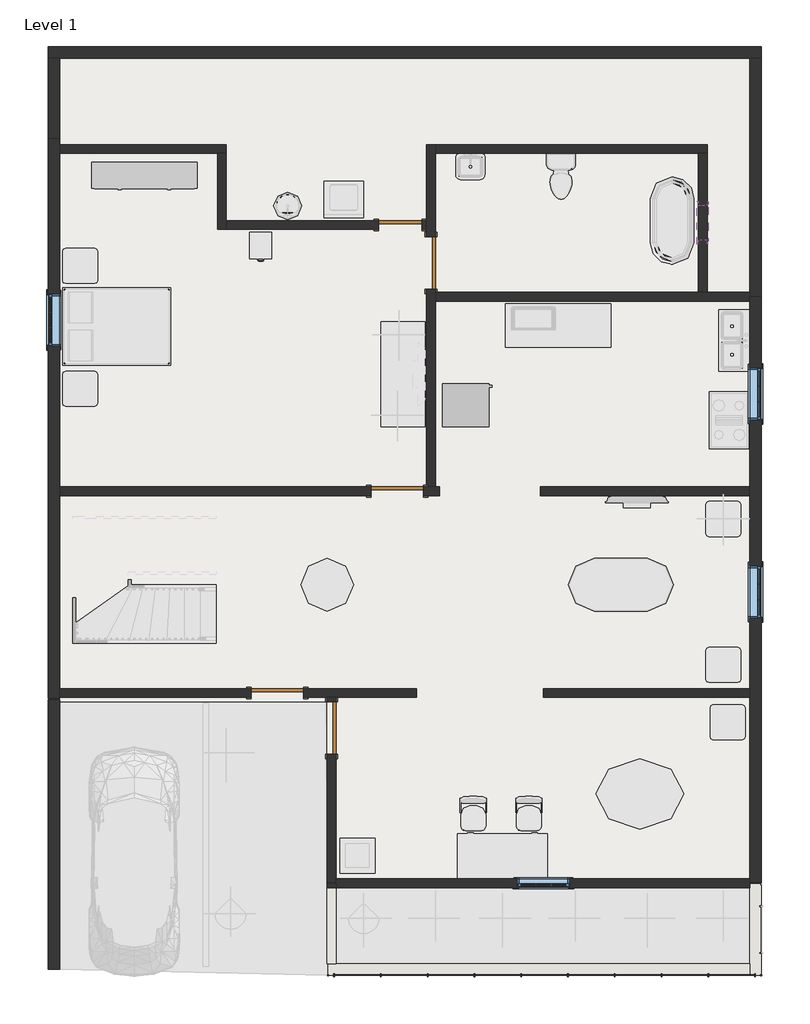
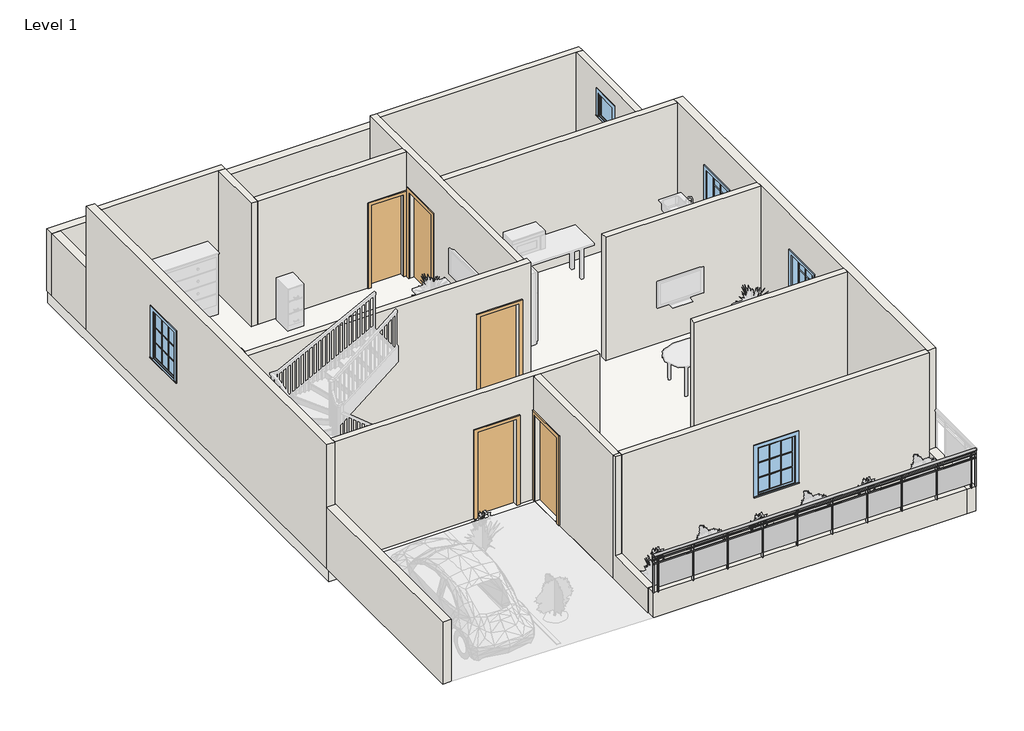
# One storey, part 1 of 3: 22 walls, 5 doors, 5 windows, 1 railing, 1 slab.
"""IFC4 building model written with IfcOpenShell, lengths in millimetres."""

from ifc_helpers import new_model, si_unit, point, frame, origin, origin_with_axes, place, context, project, spatial, polyline, ellipse_curve, trimmed, outline, extrude, faceted_brep, transform, mapped, element, save
from ifc_brep_helpers import plane_surface, extruded_surface, advanced_brep
from components import door_059fdd7e, door_16372e1c, door_686f89d2, window_5c190c7e, window_29c06734, window_3d781103

model = new_model("IFC4")

# Units and contexts
model_context = context("Model", 3, world=origin())
ifc_project = project(units=[si_unit("LENGTHUNIT", "METRE", prefix="MILLI")], contexts=[model_context])

# Site, building, storey
site = spatial("IfcSite", under=ifc_project)
building = spatial("IfcBuilding", under=site)
storey = spatial("IfcBuildingStorey", under=building, Name="Level 1", Elevation=0.0)

# Doors
placement = place(None, origin())
door_shape = door_059fdd7e(model_context)
element("IfcDoor", 1, ObjectType="Single-Flush : 30\" x 80\"", at=placement, inside=storey, context=model_context, shape_type="MappedRepresentation", body=[
    mapped(door_shape, transform((-6603.4234692, 9056.6116886, 0.0), x_axis=(1.0, 0.0, 0.0), y_axis=(0.0, 1.0, 0.0), z_axis=(0.0, 0.0, 1.0))),
])
door_2_shape = door_16372e1c(model_context)
element("IfcDoor", 2, ObjectType="Single-Flush : 36\" x 84\"", at=placement, inside=storey, context=model_context, shape_type="MappedRepresentation", body=[
    mapped(door_2_shape, transform((-6654.2234692, 4433.8116886, 0.0), x_axis=(1.0, 0.0, 0.0), y_axis=(0.0, 1.0, 0.0), z_axis=(0.0, 0.0, 1.0))),
])
element("IfcDoor", 3, ObjectType="Single-Flush : 36\" x 84\"", at=placement, inside=storey, context=model_context, shape_type="MappedRepresentation", body=[
    mapped(door_2_shape, transform((-6070.0234692, 8396.2116886, 0.0), x_axis=(0.0, -1.0, 0.0), y_axis=(1.0, 0.0, 0.0), z_axis=(0.0, 0.0, 1.0))),
])
element("IfcDoor", 4, ObjectType="Single-Flush : 36\" x 84\"", at=placement, inside=storey, context=model_context, shape_type="MappedRepresentation", body=[
    mapped(door_2_shape, transform((-8737.0234692, 928.6116886, 0.0), x_axis=(1.0, 0.0, 0.0), y_axis=(0.0, 1.0, 0.0), z_axis=(0.0, 0.0, 1.0))),
])
door_3_shape = door_686f89d2(model_context)
element("IfcDoor", 5, ObjectType="Single-Flush : 36\" x 84\"", at=placement, inside=storey, context=model_context, shape_type="MappedRepresentation", body=[
    mapped(door_3_shape, transform((-7797.2234692, 319.0116886, 0.0), x_axis=(0.0, 1.0, 0.0), y_axis=(-1.0, 0.0, 0.0), z_axis=(0.0, 0.0, 1.0))),
])

# Railing
element("IfcRailing", 6, ObjectType="Glass Panel - Bottom Fill", at=placement, inside=storey, context=model_context, shape_type="SolidModel", body=[
    advanced_brep(
    [(-7860.7234692, -3935.4883114, 1524.0), (-7860.7234692, -4011.6883114, 1524.0), (-329.6234692, -3935.4883114, 1524.0), (-329.6234692, -4011.6883114, 1524.0)],
    [
        (0, 1, ellipse_curve(frame((-7860.7234692, -3973.5883114, 1524.0), z_axis=(-1.0, 0.0, 0.0), x_axis=(0.0, -1.0, 0.0)), 38.1, 28.575)),
        (1, 0, ellipse_curve(frame((-7860.7234692, -3973.5883114, 1524.0), z_axis=(-1.0, 0.0, 0.0), x_axis=(0.0, -1.0, 0.0)), 38.1, 28.575)),
        (2, 3, ellipse_curve(frame((-329.6234692, -3973.5883114, 1524.0), z_axis=(1.0, 0.0, 0.0), x_axis=(0.0, -1.0, 0.0)), 38.1, 28.575)),
        (3, 2, ellipse_curve(frame((-329.6234692, -3973.5883114, 1524.0), z_axis=(1.0, 0.0, 0.0), x_axis=(0.0, -1.0, 0.0)), 38.1, 28.575)),
        (0, 2),
        (3, 1),
    ],
    [
        plane_surface(frame((-7860.7234692, -3973.5883114, 1524.0), z_axis=(-1.0, 0.0, 0.0), x_axis=(0.0, 1.0, 0.0))),
        plane_surface(frame((-329.6234692, -3973.5883114, 1524.0), z_axis=(1.0, 0.0, 0.0), x_axis=(0.0, 1.0, 0.0))),
        extruded_surface(trimmed(ellipse_curve(frame((-329.6234692, -3973.5883114, 1524.0), z_axis=(-1.0, 0.0, 0.0), x_axis=(0.0, -1.0, 0.0)), 38.1, 28.575), [point((-329.6234692, -3935.4883114, 1524.0))], [point((-329.6234692, -4011.6883114, 1524.0))], True, "CARTESIAN"), (-7531.1, 0.0, 0.0), 7531.1),
        extruded_surface(trimmed(ellipse_curve(frame((-329.6234692, -3973.5883114, 1524.0), z_axis=(-1.0, 0.0, 0.0), x_axis=(0.0, -1.0, 0.0)), 38.1, 28.575), [point((-329.6234692, -4011.6883114, 1524.0))], [point((-329.6234692, -3935.4883114, 1524.0))], True, "CARTESIAN"), (-7531.1, 0.0, 0.0), 7531.1),
    ],
    [
        (0, [[1, 2]]),
        (1, [[3, 4]]),
        (2, [[-1, 5, -4, 6]]),
        (3, [[-2, -6, -3, -5]]),
    ],
),
    extrude(outline(polyline([(-7860.7234692, -3986.2883114), (-7860.7234692, -3960.8883114), (-329.6234692, -3960.8883114), (-329.6234692, -3986.2883114), (-7860.7234692, -3986.2883114)])), frame((0.0, 0.0, 1409.7), z_axis=(0.0, 0.0, 1.0), x_axis=(1.0, 0.0, 0.0)), (0.0, 0.0, 1.0), 25.4),
    extrude(outline(polyline([(-7860.7234692, -3986.2883114), (-7860.7234692, -3960.8883114), (-329.6234692, -3960.8883114), (-329.6234692, -3986.2883114), (-7860.7234692, -3986.2883114)])), frame((0.0, 0.0, 1308.1), z_axis=(0.0, 0.0, 1.0), x_axis=(1.0, 0.0, 0.0)), (0.0, 0.0, 1.0), 25.4),
    extrude(outline(polyline([(-443.9234692, -3998.9883114), (-443.9234692, -3948.1883114), (-431.2234692, -3948.1883114), (-431.2234692, -3998.9883114), (-443.9234692, -3998.9883114)])), frame((0.0, 0.0, 609.6), z_axis=(0.0, 0.0, 1.0), x_axis=(1.0, 0.0, 0.0)), (0.0, 0.0, 1.0), 885.6788223),
    extrude(outline(polyline([(-1250.3734692, -3967.0531544), (-437.5734692, -3967.0531544), (-437.5734692, -3973.4031544), (-1250.3734692, -3973.4031544), (-1250.3734692, -3967.0531544)])), frame((0.0, 0.0, 711.2), z_axis=(0.0, 0.0, 1.0), x_axis=(1.0, 0.0, 0.0)), (0.0, 0.0, 1.0), 596.9),
    extrude(outline(polyline([(-1256.7234692, -3998.9883114), (-1256.7234692, -3948.1883114), (-1244.0234692, -3948.1883114), (-1244.0234692, -3998.9883114), (-1256.7234692, -3998.9883114)])), frame((0.0, 0.0, 609.6), z_axis=(0.0, 0.0, 1.0), x_axis=(1.0, 0.0, 0.0)), (0.0, 0.0, 1.0), 885.6788223),
    extrude(outline(polyline([(-2063.1734692, -3967.0531544), (-1250.3734692, -3967.0531544), (-1250.3734692, -3973.4031544), (-2063.1734692, -3973.4031544), (-2063.1734692, -3967.0531544)])), frame((0.0, 0.0, 711.2), z_axis=(0.0, 0.0, 1.0), x_axis=(1.0, 0.0, 0.0)), (0.0, 0.0, 1.0), 596.9),
    extrude(outline(polyline([(-2069.5234692, -3998.9883114), (-2069.5234692, -3948.1883114), (-2056.8234692, -3948.1883114), (-2056.8234692, -3998.9883114), (-2069.5234692, -3998.9883114)])), frame((0.0, 0.0, 609.6), z_axis=(0.0, 0.0, 1.0), x_axis=(1.0, 0.0, 0.0)), (0.0, 0.0, 1.0), 885.6788223),
    extrude(outline(polyline([(-2875.9734692, -3967.0531544), (-2063.1734692, -3967.0531544), (-2063.1734692, -3973.4031544), (-2875.9734692, -3973.4031544), (-2875.9734692, -3967.0531544)])), frame((0.0, 0.0, 711.2), z_axis=(0.0, 0.0, 1.0), x_axis=(1.0, 0.0, 0.0)), (0.0, 0.0, 1.0), 596.9),
    extrude(outline(polyline([(-2882.3234692, -3998.9883114), (-2882.3234692, -3948.1883114), (-2869.6234692, -3948.1883114), (-2869.6234692, -3998.9883114), (-2882.3234692, -3998.9883114)])), frame((0.0, 0.0, 609.6), z_axis=(0.0, 0.0, 1.0), x_axis=(1.0, 0.0, 0.0)), (0.0, 0.0, 1.0), 885.6788223),
    extrude(outline(polyline([(-3688.7734692, -3967.0531544), (-2875.9734692, -3967.0531544), (-2875.9734692, -3973.4031544), (-3688.7734692, -3973.4031544), (-3688.7734692, -3967.0531544)])), frame((0.0, 0.0, 711.2), z_axis=(0.0, 0.0, 1.0), x_axis=(1.0, 0.0, 0.0)), (0.0, 0.0, 1.0), 596.9),
    extrude(outline(polyline([(-3695.1234692, -3998.9883114), (-3695.1234692, -3948.1883114), (-3682.4234692, -3948.1883114), (-3682.4234692, -3998.9883114), (-3695.1234692, -3998.9883114)])), frame((0.0, 0.0, 609.6), z_axis=(0.0, 0.0, 1.0), x_axis=(1.0, 0.0, 0.0)), (0.0, 0.0, 1.0), 885.6788223),
    extrude(outline(polyline([(-4501.5734692, -3967.0531544), (-3688.7734692, -3967.0531544), (-3688.7734692, -3973.4031544), (-4501.5734692, -3973.4031544), (-4501.5734692, -3967.0531544)])), frame((0.0, 0.0, 711.2), z_axis=(0.0, 0.0, 1.0), x_axis=(1.0, 0.0, 0.0)), (0.0, 0.0, 1.0), 596.9),
    extrude(outline(polyline([(-4507.9234692, -3998.9883114), (-4507.9234692, -3948.1883114), (-4495.2234692, -3948.1883114), (-4495.2234692, -3998.9883114), (-4507.9234692, -3998.9883114)])), frame((0.0, 0.0, 609.6), z_axis=(0.0, 0.0, 1.0), x_axis=(1.0, 0.0, 0.0)), (0.0, 0.0, 1.0), 885.6788223),
    extrude(outline(polyline([(-5314.3734692, -3967.0531544), (-4501.5734692, -3967.0531544), (-4501.5734692, -3973.4031544), (-5314.3734692, -3973.4031544), (-5314.3734692, -3967.0531544)])), frame((0.0, 0.0, 711.2), z_axis=(0.0, 0.0, 1.0), x_axis=(1.0, 0.0, 0.0)), (0.0, 0.0, 1.0), 596.9),
    extrude(outline(polyline([(-5320.7234692, -3998.9883114), (-5320.7234692, -3948.1883114), (-5308.0234692, -3948.1883114), (-5308.0234692, -3998.9883114), (-5320.7234692, -3998.9883114)])), frame((0.0, 0.0, 609.6), z_axis=(0.0, 0.0, 1.0), x_axis=(1.0, 0.0, 0.0)), (0.0, 0.0, 1.0), 885.6788223),
    extrude(outline(polyline([(-6127.1734692, -3967.0531544), (-5314.3734692, -3967.0531544), (-5314.3734692, -3973.4031544), (-6127.1734692, -3973.4031544), (-6127.1734692, -3967.0531544)])), frame((0.0, 0.0, 711.2), z_axis=(0.0, 0.0, 1.0), x_axis=(1.0, 0.0, 0.0)), (0.0, 0.0, 1.0), 596.9),
    extrude(outline(polyline([(-6133.5234692, -3998.9883114), (-6133.5234692, -3948.1883114), (-6120.8234692, -3948.1883114), (-6120.8234692, -3998.9883114), (-6133.5234692, -3998.9883114)])), frame((0.0, 0.0, 609.6), z_axis=(0.0, 0.0, 1.0), x_axis=(1.0, 0.0, 0.0)), (0.0, 0.0, 1.0), 885.6788223),
    extrude(outline(polyline([(-6939.9734692, -3967.0531544), (-6127.1734692, -3967.0531544), (-6127.1734692, -3973.4031544), (-6939.9734692, -3973.4031544), (-6939.9734692, -3967.0531544)])), frame((0.0, 0.0, 711.2), z_axis=(0.0, 0.0, 1.0), x_axis=(1.0, 0.0, 0.0)), (0.0, 0.0, 1.0), 596.9),
    extrude(outline(polyline([(-6946.3234692, -3998.9883114), (-6946.3234692, -3948.1883114), (-6933.6234692, -3948.1883114), (-6933.6234692, -3998.9883114), (-6946.3234692, -3998.9883114)])), frame((0.0, 0.0, 609.6), z_axis=(0.0, 0.0, 1.0), x_axis=(1.0, 0.0, 0.0)), (0.0, 0.0, 1.0), 885.6788223),
    extrude(outline(polyline([(-7752.7734692, -3967.0531544), (-6939.9734692, -3967.0531544), (-6939.9734692, -3973.4031544), (-7752.7734692, -3973.4031544), (-7752.7734692, -3967.0531544)])), frame((0.0, 0.0, 711.2), z_axis=(0.0, 0.0, 1.0), x_axis=(1.0, 0.0, 0.0)), (0.0, 0.0, 1.0), 596.9),
    extrude(outline(polyline([(-7759.1234692, -3998.9883114), (-7759.1234692, -3948.1883114), (-7746.4234692, -3948.1883114), (-7746.4234692, -3998.9883114), (-7759.1234692, -3998.9883114)])), frame((0.0, 0.0, 609.6), z_axis=(0.0, 0.0, 1.0), x_axis=(1.0, 0.0, 0.0)), (0.0, 0.0, 1.0), 885.6788223),
    extrude(outline(polyline([(-342.3234692, -3983.1133114), (-342.3234692, -3964.0633114), (-323.2734692, -3964.0633114), (-323.2734692, -3983.1133114), (-342.3234692, -3983.1133114)])), frame((0.0, 0.0, 609.6), z_axis=(0.0, 0.0, 1.0), x_axis=(1.0, 0.0, 0.0)), (0.0, 0.0, 1.0), 885.6788223),
    extrude(outline(polyline([(-7867.0734692, -3983.1133114), (-7867.0734692, -3964.0633114), (-7848.0234692, -3964.0633114), (-7848.0234692, -3983.1133114), (-7867.0734692, -3983.1133114)])), frame((0.0, 0.0, 609.6), z_axis=(0.0, 0.0, 1.0), x_axis=(1.0, 0.0, 0.0)), (0.0, 0.0, 1.0), 885.6788223),
])

# Slab
element("IfcSlab", 7, ObjectType="Generic - 12\"", at=placement, inside=storey, context=model_context, shape_type="SweptSolid", body=[
    extrude(outline(polyline([(-329.6234692, 12155.4116886), (-329.6234692, -2449.5883114), (-7873.4234692, -2449.5883114), (-7873.4234692, 776.2116886), (-12699.4234692, 776.2116886), (-12699.4234692, 12155.4116886), (-329.6234692, 12155.4116886)])), frame((0.0, 0.0, -304.8), z_axis=(0.0, 0.0, 1.0), x_axis=(1.0, 0.0, 0.0)), (0.0, 0.0, 1.0), 304.8),
])

# Walls
element("IfcWall", 8, ObjectType="Generic - 8\"", at=placement, inside=storey, context=model_context, shape_type="Brep", body=[
    faceted_brep([(-12724.8234692, 11952.2116886, 0.0), (-12521.6234692, 11952.2116886, 0.0), (-532.8234692, 11952.2116886, 0.0), (-329.6234692, 11952.2116886, 0.0), (-329.6234692, 11952.2116886, 1524.0), (-532.8234692, 11952.2116886, 1524.0), (-12521.6234692, 11952.2116886, 1524.0), (-12724.8234692, 11952.2116886, 1524.0), (-12724.8234692, 12155.4116886, 0.0), (-12724.8234692, 12155.4116886, 1524.0), (-329.6234692, 12155.4116886, 1524.0), (-329.6234692, 12155.4116886, 0.0)], [[[0, 1, 2, 3, 4, 5, 6, 7]], [[8, 9, 10, 11]], [[3, 2, 1, 0, 8, 11]], [[7, 6, 5, 4, 10, 9]], [[4, 3, 11, 10]], [[0, 7, 9, 8]]]),
])
element("IfcWall", 9, ObjectType="Generic - 8\"", at=placement, inside=storey, context=model_context, shape_type="Brep", body=[
    faceted_brep([(-532.8234692, 11952.2116886, 0.0), (-532.8234692, 7888.2116886, 0.0), (-532.8234692, 7812.0116886, 0.0), (-532.8234692, 7812.0116886, 1524.0), (-532.8234692, 11952.2116886, 1524.0), (-329.6234692, 11952.2116886, 0.0), (-329.6234692, 11952.2116886, 1524.0), (-329.6234692, 7812.0116886, 1524.0), (-329.6234692, 7812.0116886, 0.0)], [[[0, 1, 2, 3, 4]], [[5, 6, 7, 8]], [[2, 1, 0, 5, 8]], [[3, 2, 8, 7]], [[4, 3, 7, 6]], [[0, 4, 6, 5]]]),
])
element("IfcWall", 10, ObjectType="Generic - 8\"", at=placement, inside=storey, context=model_context, shape_type="Brep", body=[
    faceted_brep([(-532.8234692, -3770.3883114, 0.0), (-7721.0234692, -3770.3883114, 0.0), (-7860.7234692, -3770.3883114, 0.0), (-7860.7234692, -3770.3883114, 609.6), (-7721.0234692, -3770.3883114, 609.6), (-532.8234692, -3770.3883114, 609.6), (-532.8234692, -3973.5883114, 0.0), (-532.8234692, -3973.5883114, 609.6), (-7860.7234692, -3973.5883114, 609.6), (-7860.7234692, -3973.5883114, 0.0)], [[[0, 1, 2, 3, 4, 5]], [[6, 7, 8, 9]], [[2, 1, 0, 6, 9]], [[3, 2, 9, 8]], [[5, 4, 3, 8, 7]], [[0, 5, 7, 6]]]),
])
element("IfcWall", 11, ObjectType="Generic - 8\"", at=placement, inside=storey, context=model_context, shape_type="SweptSolid", body=[
    extrude(outline(polyline([(-12521.6234692, 814.3116886), (-12521.6234692, -3871.9883114), (-12724.8234692, -3871.9883114), (-12724.8234692, 814.3116886), (-12521.6234692, 814.3116886)])), origin_with_axes(), (0.0, 0.0, 1.0), 1524.0),
])
element("IfcWall", 12, ObjectType="Generic - 8\"", at=placement, inside=storey, context=model_context, shape_type="Brep", body=[
    faceted_brep([(-532.8234692, -2386.0883114, 0.0), (-532.8234692, -2449.5883114, 0.0), (-532.8234692, -3770.3883114, 0.0), (-532.8234692, -3973.5883114, 0.0), (-532.8234692, -3973.5883114, 609.6), (-532.8234692, -3770.3883114, 609.6), (-532.8234692, -2386.0883114, 609.6), (-329.6234692, -2386.0883114, 0.0), (-329.6234692, -2386.0883114, 609.6), (-329.6234692, -3973.5883114, 609.6), (-329.6234692, -3973.5883114, 0.0)], [[[0, 1, 2, 3, 4, 5, 6]], [[7, 8, 9, 10]], [[3, 2, 1, 0, 7, 10]], [[6, 5, 4, 9, 8]], [[0, 6, 8, 7]], [[4, 3, 10, 9]]]),
])
element("IfcWall", 13, ObjectType="Generic - 8\"", at=placement, inside=storey, context=model_context, shape_type="SweptSolid", body=[
    extrude(outline(polyline([(-12521.6234692, 11952.2116886), (-12521.6234692, 10555.2116886), (-12724.8234692, 10555.2116886), (-12724.8234692, 11952.2116886), (-12521.6234692, 11952.2116886)])), origin_with_axes(), (0.0, 0.0, 1.0), 1524.0),
])
element("IfcWall", 14, ObjectType="Generic - 8\" 2", at=placement, inside=storey, context=model_context, shape_type="Brep", body=[
    faceted_brep([(-12521.6234692, 839.7116886, 0.0), (-12521.6234692, 852.4116886, 0.0), (-12521.6234692, 1004.8116886, 0.0), (-12521.6234692, 4357.6116886, 0.0), (-12521.6234692, 4510.0116886, 0.0), (-12521.6234692, 10301.2116886, 0.0), (-12521.6234692, 10453.6116886, 0.0), (-12521.6234692, 10555.2116886, 0.0), (-12521.6234692, 10555.2116886, 3048.0), (-12521.6234692, 10453.6116886, 3048.0), (-12521.6234692, 10301.2116886, 3048.0), (-12521.6234692, 4510.0116886, 3048.0), (-12521.6234692, 4357.6116886, 3048.0), (-12521.6234692, 1004.8116886, 3048.0), (-12521.6234692, 852.4116886, 3048.0), (-12521.6234692, 839.7116886, 3048.0), (-12521.6234692, 7862.8116886, 2133.6), (-12521.6234692, 7862.8116886, 914.4), (-12521.6234692, 6948.4116886, 914.4), (-12521.6234692, 6948.4116886, 2133.6), (-12724.8234692, 839.7116886, 0.0), (-12724.8234692, 839.7116886, 3048.0), (-12724.8234692, 10555.2116886, 3048.0), (-12724.8234692, 10555.2116886, 0.0), (-12724.8234692, 7862.8116886, 2133.6), (-12724.8234692, 6948.4116886, 2133.6), (-12724.8234692, 6948.4116886, 914.4), (-12724.8234692, 7862.8116886, 914.4)], [[[0, 1, 2, 3, 4, 5, 6, 7, 8, 9, 10, 11, 12, 13, 14, 15], [16, 17, 18, 19]], [[20, 21, 22, 23], [24, 25, 26, 27]], [[7, 6, 5, 4, 3, 2, 1, 0, 20, 23]], [[8, 7, 23, 22]], [[0, 15, 21, 20]], [[17, 16, 24, 27]], [[18, 17, 27, 26]], [[19, 18, 26, 25]], [[16, 19, 25, 24]], [[15, 14, 13, 12, 11, 10, 9, 8, 22, 21]]]),
])
element("IfcWall", 15, ObjectType="Generic - 8\" 2", at=placement, inside=storey, context=model_context, shape_type="Brep", body=[
    faceted_brep([(-532.8234692, 7812.0116886, 0.0), (-532.8234692, 7735.8116886, 0.0), (-532.8234692, 4510.0116886, 0.0), (-532.8234692, 4357.6116886, 0.0), (-532.8234692, 1004.8116886, 0.0), (-532.8234692, 852.4116886, 0.0), (-532.8234692, -2360.6883114, 0.0), (-532.8234692, -2360.6883114, 3048.0), (-532.8234692, 852.4116886, 3048.0), (-532.8234692, 1004.8116886, 3048.0), (-532.8234692, 4357.6116886, 3048.0), (-532.8234692, 4510.0116886, 3048.0), (-532.8234692, 7735.8116886, 3048.0), (-532.8234692, 7888.2116886, 3048.0), (-532.8234692, 7888.2116886, 1524.0), (-532.8234692, 7812.0116886, 1524.0), (-532.8234692, 5665.7116886, 2133.6), (-532.8234692, 5665.7116886, 914.4), (-532.8234692, 6580.1116886, 914.4), (-532.8234692, 6580.1116886, 2133.6), (-532.8234692, 2224.0116886, 2133.6), (-532.8234692, 2224.0116886, 914.4), (-532.8234692, 3138.4116886, 914.4), (-532.8234692, 3138.4116886, 2133.6), (-329.6234692, 7812.0116886, 0.0), (-329.6234692, 7812.0116886, 1524.0), (-329.6234692, 7888.2116886, 1524.0), (-329.6234692, 7888.2116886, 3048.0), (-329.6234692, -2360.6883114, 3048.0), (-329.6234692, -2360.6883114, 0.0), (-329.6234692, 5665.7116886, 2133.6), (-329.6234692, 6580.1116886, 2133.6), (-329.6234692, 6580.1116886, 914.4), (-329.6234692, 5665.7116886, 914.4), (-329.6234692, 2224.0116886, 2133.6), (-329.6234692, 3138.4116886, 2133.6), (-329.6234692, 3138.4116886, 914.4), (-329.6234692, 2224.0116886, 914.4)], [[[0, 1, 2, 3, 4, 5, 6, 7, 8, 9, 10, 11, 12, 13, 14, 15], [16, 17, 18, 19], [20, 21, 22, 23]], [[24, 25, 26, 27, 28, 29], [30, 31, 32, 33], [34, 35, 36, 37]], [[6, 5, 4, 3, 2, 1, 0, 24, 29]], [[7, 6, 29, 28]], [[0, 15, 25, 24]], [[14, 26, 25, 15]], [[14, 13, 27, 26]], [[17, 16, 30, 33]], [[18, 17, 33, 32]], [[19, 18, 32, 31]], [[16, 19, 31, 30]], [[21, 20, 34, 37]], [[22, 21, 37, 36]], [[23, 22, 36, 35]], [[20, 23, 35, 34]], [[13, 12, 11, 10, 9, 8, 7, 28, 27]]]),
])
element("IfcWall", 16, ObjectType="INNER 6\"", at=placement, inside=storey, context=model_context, shape_type="Brep", body=[
    faceted_brep([(-12521.6234692, 10301.2116886, 0.0), (-9778.4234692, 10301.2116886, 0.0), (-9626.0234692, 10301.2116886, 0.0), (-9626.0234692, 10301.2116886, 3048.0), (-9778.4234692, 10301.2116886, 3048.0), (-12521.6234692, 10301.2116886, 3048.0), (-12521.6234692, 10453.6116886, 0.0), (-12521.6234692, 10453.6116886, 3048.0), (-9626.0234692, 10453.6116886, 3048.0), (-9626.0234692, 10453.6116886, 0.0)], [[[0, 1, 2, 3, 4, 5]], [[6, 7, 8, 9]], [[2, 1, 0, 6, 9]], [[0, 5, 7, 6]], [[3, 2, 9, 8]], [[5, 4, 3, 8, 7]]]),
])
element("IfcWall", 17, ObjectType="INNER 6\"", at=placement, inside=storey, context=model_context, shape_type="Brep", body=[
    faceted_brep([(-9778.4234692, 10301.2116886, 0.0), (-9778.4234692, 8980.4116886, 0.0), (-9778.4234692, 8980.4116886, 3048.0), (-9778.4234692, 10301.2116886, 3048.0), (-9626.0234692, 10301.2116886, 0.0), (-9626.0234692, 10301.2116886, 3048.0), (-9626.0234692, 9132.8116886, 3048.0), (-9626.0234692, 8980.4116886, 3048.0), (-9626.0234692, 8980.4116886, 0.0), (-9626.0234692, 9132.8116886, 0.0)], [[[0, 1, 2, 3]], [[4, 5, 6, 7, 8, 9]], [[1, 0, 4, 9, 8]], [[0, 3, 5, 4]], [[2, 1, 8, 7]], [[3, 2, 7, 6, 5]]]),
])
element("IfcWall", 18, ObjectType="INNER 6\"", at=placement, inside=storey, context=model_context, shape_type="SweptSolid", body=[
    extrude(outline(polyline([(3048.0, -9626.0234692), (0.0, -9626.0234692), (0.0, -6984.4234692), (2032.0, -6984.4234692), (2032.0, -6222.4234692), (0.0, -6222.4234692), (0.0, -6146.2234692), (3048.0, -6146.2234692), (3048.0, -9626.0234692)])), frame((0.0, 8980.4116886, 0.0), z_axis=(0.0, 1.0, 0.0), x_axis=(0.0, 0.0, 1.0)), (0.0, 0.0, 1.0), 152.4),
])
element("IfcWall", 19, ObjectType="INNER 6\"", at=placement, inside=storey, context=model_context, shape_type="Brep", body=[
    faceted_brep([(-5993.8234692, 4510.0116886, 0.0), (-5993.8234692, 7735.8116886, 0.0), (-5993.8234692, 7888.2116886, 0.0), (-5993.8234692, 7939.0116886, 0.0), (-5993.8234692, 7939.0116886, 2133.6), (-5993.8234692, 8853.4116886, 2133.6), (-5993.8234692, 8853.4116886, 0.0), (-5993.8234692, 10301.2116886, 0.0), (-5993.8234692, 10453.6116886, 0.0), (-5993.8234692, 10453.6116886, 3048.0), (-5993.8234692, 10301.2116886, 3048.0), (-5993.8234692, 7888.2116886, 3048.0), (-5993.8234692, 7735.8116886, 3048.0), (-5993.8234692, 4510.0116886, 3048.0), (-6146.2234692, 7939.0116886, 2133.6), (-6146.2234692, 7939.0116886, 0.0), (-6146.2234692, 4510.0116886, 0.0), (-6146.2234692, 4510.0116886, 3048.0), (-6146.2234692, 8980.4116886, 3048.0), (-6146.2234692, 9132.8116886, 3048.0), (-6146.2234692, 10453.6116886, 3048.0), (-6146.2234692, 10453.6116886, 0.0), (-6146.2234692, 9132.8116886, 0.0), (-6146.2234692, 8980.4116886, 0.0), (-6146.2234692, 8853.4116886, 0.0), (-6146.2234692, 8853.4116886, 2133.6)], [[[0, 1, 2, 3, 4, 5, 6, 7, 8, 9, 10, 11, 12, 13]], [[14, 15, 16, 17, 18, 19, 20, 21, 22, 23, 24, 25]], [[16, 15, 3, 2, 1, 0]], [[24, 23, 22, 21, 8, 7, 6]], [[9, 8, 21, 20]], [[0, 13, 17, 16]], [[4, 3, 15, 14]], [[5, 4, 14, 25]], [[6, 5, 25, 24]], [[13, 12, 11, 10, 9, 20, 19, 18, 17]]]),
])
element("IfcWall", 20, ObjectType="INNER 6\"", at=placement, inside=storey, context=model_context, shape_type="Brep", body=[
    faceted_brep([(-5993.8234692, 10301.2116886, 0.0), (-1421.8234692, 10301.2116886, 0.0), (-1269.4234692, 10301.2116886, 0.0), (-1269.4234692, 10301.2116886, 3048.0), (-1421.8234692, 10301.2116886, 3048.0), (-5993.8234692, 10301.2116886, 3048.0), (-5993.8234692, 10453.6116886, 0.0), (-5993.8234692, 10453.6116886, 3048.0), (-1269.4234692, 10453.6116886, 3048.0), (-1269.4234692, 10453.6116886, 0.0)], [[[0, 1, 2, 3, 4, 5]], [[6, 7, 8, 9]], [[2, 1, 0, 6, 9]], [[0, 5, 7, 6]], [[3, 2, 9, 8]], [[5, 4, 3, 8, 7]]]),
])
element("IfcWall", 21, ObjectType="INNER 6\"", at=placement, inside=storey, context=model_context, shape_type="SweptSolid", body=[
    extrude(outline(polyline([(10301.2116886, 0.0), (7888.2116886, 0.0), (7888.2116886, 3048.0), (10301.2116886, 3048.0), (10301.2116886, 0.0)]), holes=[polyline([(9399.5116886, 2616.2), (8789.9116886, 2616.2), (8789.9116886, 2006.6), (9399.5116886, 2006.6), (9399.5116886, 2616.2)])]), frame((-1421.8234692, 0.0, 0.0), z_axis=(1.0, 0.0, 0.0), x_axis=(0.0, 1.0, 0.0)), (0.0, 0.0, 1.0), 152.4),
])
element("IfcWall", 22, ObjectType="INNER 6\"", at=placement, inside=storey, context=model_context, shape_type="Brep", body=[
    faceted_brep([(-5993.8234692, 7735.8116886, 0.0), (-532.8234692, 7735.8116886, 0.0), (-532.8234692, 7735.8116886, 3048.0), (-5993.8234692, 7735.8116886, 3048.0), (-5993.8234692, 7888.2116886, 0.0), (-5993.8234692, 7888.2116886, 3048.0), (-1421.8234692, 7888.2116886, 3048.0), (-1269.4234692, 7888.2116886, 3048.0), (-532.8234692, 7888.2116886, 3048.0), (-532.8234692, 7888.2116886, 1524.0), (-532.8234692, 7888.2116886, 0.0), (-1269.4234692, 7888.2116886, 0.0), (-1421.8234692, 7888.2116886, 0.0), (-532.8234692, 7812.0116886, 0.0)], [[[0, 1, 2, 3]], [[4, 5, 6, 7, 8, 9, 10, 11, 12]], [[1, 0, 4, 12, 11, 10, 13]], [[0, 3, 5, 4]], [[1, 13, 10, 9, 8, 2]], [[3, 2, 8, 7, 6, 5]]]),
])
element("IfcWall", 23, ObjectType="INNER 6\"", at=placement, inside=storey, context=model_context, shape_type="SweptSolid", body=[
    extrude(outline(polyline([(-4165.0234692, 4510.0116886), (-532.8234692, 4510.0116886), (-532.8234692, 4357.6116886), (-4165.0234692, 4357.6116886), (-4165.0234692, 4510.0116886)])), origin_with_axes(), (0.0, 0.0, 1.0), 3048.0),
])
element("IfcWall", 24, ObjectType="INNER 6\"", at=placement, inside=storey, context=model_context, shape_type="Brep", body=[
    faceted_brep([(-8279.8234692, 852.4116886, 2133.6), (-8279.8234692, 852.4116886, 0.0), (-7873.4234692, 852.4116886, 0.0), (-7721.0234692, 852.4116886, 0.0), (-6324.0234692, 852.4116886, 0.0), (-6324.0234692, 852.4116886, 3048.0), (-7721.0234692, 852.4116886, 3048.0), (-7873.4234692, 852.4116886, 3048.0), (-12521.6234692, 852.4116886, 3048.0), (-12521.6234692, 852.4116886, 0.0), (-9194.2234692, 852.4116886, 0.0), (-9194.2234692, 852.4116886, 2133.6), (-6324.0234692, 1004.8116886, 0.0), (-8279.8234692, 1004.8116886, 0.0), (-8279.8234692, 1004.8116886, 2133.6), (-9194.2234692, 1004.8116886, 2133.6), (-9194.2234692, 1004.8116886, 0.0), (-12521.6234692, 1004.8116886, 0.0), (-12521.6234692, 1004.8116886, 3048.0), (-6324.0234692, 1004.8116886, 3048.0)], [[[0, 1, 2, 3, 4, 5, 6, 7, 8, 9, 10, 11]], [[12, 13, 14, 15, 16, 17, 18, 19]], [[10, 9, 17, 16]], [[4, 3, 2, 1, 13, 12]], [[5, 4, 12, 19]], [[9, 8, 18, 17]], [[14, 13, 1, 0]], [[15, 14, 0, 11]], [[16, 15, 11, 10]], [[8, 7, 6, 5, 19, 18]]]),
])
element("IfcWall", 25, ObjectType="INNER 6\"", at=placement, inside=storey, context=model_context, shape_type="Brep", body=[
    faceted_brep([(-7873.4234692, 852.4116886, 0.0), (-7873.4234692, 776.2116886, 0.0), (-7873.4234692, 776.2116886, 2133.6), (-7873.4234692, -138.1883114, 2133.6), (-7873.4234692, -138.1883114, 0.0), (-7873.4234692, -2373.3883114, 0.0), (-7873.4234692, -2373.3883114, 3048.0), (-7873.4234692, 776.2116886, 3048.0), (-7873.4234692, 852.4116886, 3048.0), (-7721.0234692, 776.2116886, 2133.6), (-7721.0234692, 776.2116886, 0.0), (-7721.0234692, 852.4116886, 0.0), (-7721.0234692, 852.4116886, 3048.0), (-7721.0234692, -2297.1883114, 3048.0), (-7721.0234692, -2373.3883114, 3048.0), (-7721.0234692, -2373.3883114, 0.0), (-7721.0234692, -2297.1883114, 0.0), (-7721.0234692, -138.1883114, 0.0), (-7721.0234692, -138.1883114, 2133.6)], [[[0, 1, 2, 3, 4, 5, 6, 7, 8]], [[9, 10, 11, 12, 13, 14, 15, 16, 17, 18]], [[11, 10, 1, 0]], [[17, 16, 15, 5, 4]], [[6, 5, 15, 14]], [[0, 8, 12, 11]], [[2, 1, 10, 9]], [[3, 2, 9, 18]], [[4, 3, 18, 17]], [[8, 7, 6, 14, 13, 12]]]),
])
element("IfcWall", 26, ObjectType="INNER 6\"", at=placement, inside=storey, context=model_context, shape_type="Brep", body=[
    faceted_brep([(-7721.0234692, -2449.5883114, 0.0), (-532.8234692, -2449.5883114, 0.0), (-532.8234692, -2449.5883114, 3048.0), (-7721.0234692, -2449.5883114, 3048.0), (-7721.0234692, -2449.5883114, 609.6), (-4571.4234692, -2449.5883114, 2133.6), (-3657.0234692, -2449.5883114, 2133.6), (-3657.0234692, -2449.5883114, 914.4), (-4571.4234692, -2449.5883114, 914.4), (-7721.0234692, -2297.1883114, 0.0), (-7721.0234692, -2297.1883114, 3048.0), (-532.8234692, -2297.1883114, 3048.0), (-532.8234692, -2297.1883114, 0.0), (-4571.4234692, -2297.1883114, 2133.6), (-4571.4234692, -2297.1883114, 914.4), (-3657.0234692, -2297.1883114, 914.4), (-3657.0234692, -2297.1883114, 2133.6), (-7721.0234692, -2373.3883114, 0.0), (-532.8234692, -2386.0883114, 0.0), (-7721.0234692, -2373.3883114, 3048.0)], [[[0, 1, 2, 3, 4], [5, 6, 7, 8]], [[9, 10, 11, 12], [13, 14, 15, 16]], [[1, 0, 17, 9, 12, 18]], [[0, 4, 3, 19, 10, 9, 17]], [[2, 1, 18, 12, 11]], [[14, 13, 5, 8]], [[15, 14, 8, 7]], [[16, 15, 7, 6]], [[13, 16, 6, 5]], [[3, 2, 11, 10, 19]]]),
])
element("IfcWall", 27, ObjectType="INNER 6\"", at=placement, inside=storey, context=model_context, shape_type="Brep", body=[
    faceted_brep([(-5917.6234692, 4510.0116886, 0.0), (-5993.8234692, 4510.0116886, 0.0), (-6146.2234692, 4510.0116886, 0.0), (-6197.0234692, 4510.0116886, 0.0), (-6197.0234692, 4510.0116886, 2133.6), (-7111.4234692, 4510.0116886, 2133.6), (-7111.4234692, 4510.0116886, 0.0), (-12521.6234692, 4510.0116886, 0.0), (-12521.6234692, 4510.0116886, 3048.0), (-6146.2234692, 4510.0116886, 3048.0), (-5993.8234692, 4510.0116886, 3048.0), (-5917.6234692, 4510.0116886, 3048.0), (-6197.0234692, 4357.6116886, 2133.6), (-6197.0234692, 4357.6116886, 0.0), (-5917.6234692, 4357.6116886, 0.0), (-5917.6234692, 4357.6116886, 3048.0), (-12521.6234692, 4357.6116886, 3048.0), (-12521.6234692, 4357.6116886, 0.0), (-7111.4234692, 4357.6116886, 0.0), (-7111.4234692, 4357.6116886, 2133.6)], [[[0, 1, 2, 3, 4, 5, 6, 7, 8, 9, 10, 11]], [[12, 13, 14, 15, 16, 17, 18, 19]], [[18, 17, 7, 6]], [[14, 13, 3, 2, 1, 0]], [[0, 11, 15, 14]], [[8, 7, 17, 16]], [[6, 5, 19, 18]], [[5, 4, 12, 19]], [[4, 3, 13, 12]], [[11, 10, 9, 8, 16, 15]]]),
])
element("IfcWall", 28, ObjectType="INNER 6\"", at=placement, inside=storey, context=model_context, shape_type="SweptSolid", body=[
    extrude(outline(polyline([(-532.8234692, 852.4116886), (-4114.2234692, 852.4116886), (-4114.2234692, 1004.8116886), (-532.8234692, 1004.8116886), (-532.8234692, 852.4116886)])), origin_with_axes(), (0.0, 0.0, 1.0), 3048.0),
])
element("IfcWall", 29, ObjectType="INNER 6\"", at=placement, inside=storey, context=model_context, shape_type="Brep", body=[
    faceted_brep([(-7873.4234692, -2373.3883114, 0.0), (-7873.4234692, -3770.3883114, 0.0), (-7873.4234692, -3770.3883114, 609.6), (-7873.4234692, -2449.5883114, 609.6), (-7873.4234692, -2449.5883114, 3048.0), (-7873.4234692, -2373.3883114, 3048.0), (-7721.0234692, -2373.3883114, 0.0), (-7721.0234692, -2373.3883114, 3048.0), (-7721.0234692, -2449.5883114, 3048.0), (-7721.0234692, -2449.5883114, 609.6), (-7721.0234692, -3770.3883114, 609.6), (-7721.0234692, -3770.3883114, 0.0), (-7721.0234692, -2449.5883114, 0.0), (-7860.7234692, -3770.3883114, 0.0), (-7860.7234692, -3770.3883114, 609.6)], [[[0, 1, 2, 3, 4, 5]], [[6, 7, 8, 9, 10, 11, 12]], [[1, 0, 6, 12, 11, 13]], [[0, 5, 7, 6]], [[2, 1, 13, 11, 10, 14]], [[3, 2, 14, 10, 9]], [[3, 9, 8, 4]], [[5, 4, 8, 7]]]),
])

# Windows
window_shape = window_5c190c7e(model_context)
element("IfcWindow", 30, ObjectType="Casement 3x3 with Trim : 36\" x 48\"", at=placement, inside=storey, context=model_context, shape_type="MappedRepresentation", body=[
    mapped(window_shape, transform((-4114.2234692, -2373.3883114, 0.0), x_axis=(-1.0, 0.0, 0.0), y_axis=(0.0, -1.0, 0.0), z_axis=(0.0, 0.0, 1.0))),
])
window_2_shape = window_29c06734(model_context)
element("IfcWindow", 31, ObjectType="Casement 3x3 with Trim : 36\" x 48\"", at=placement, inside=storey, context=model_context, shape_type="MappedRepresentation", body=[
    mapped(window_2_shape, transform((-12623.2234692, 7405.6116886, 0.0), x_axis=(0.0, 1.0, 0.0), y_axis=(-1.0, 0.0, 0.0), z_axis=(0.0, 0.0, 1.0))),
])
element("IfcWindow", 32, ObjectType="Casement 3x3 with Trim : 36\" x 48\"", at=placement, inside=storey, context=model_context, shape_type="MappedRepresentation", body=[
    mapped(window_2_shape, transform((-431.2234692, 6122.9116886, 0.0), x_axis=(0.0, -1.0, 0.0), y_axis=(1.0, 0.0, 0.0), z_axis=(0.0, 0.0, 1.0))),
])
element("IfcWindow", 33, ObjectType="Casement 3x3 with Trim : 36\" x 48\"", at=placement, inside=storey, context=model_context, shape_type="MappedRepresentation", body=[
    mapped(window_2_shape, transform((-431.2234692, 2681.2116886, 0.0), x_axis=(0.0, -1.0, 0.0), y_axis=(1.0, 0.0, 0.0), z_axis=(0.0, 0.0, 1.0))),
])
window_3_shape = window_3d781103(model_context)
element("IfcWindow", 34, ObjectType="Transom with Trim : 24\" x 24\"", at=placement, inside=storey, context=model_context, shape_type="MappedRepresentation", body=[
    mapped(window_3_shape, transform((-1345.6234692, 9132.8116886, -152.4), x_axis=(0.0, 1.0, 0.0), y_axis=(-1.0, 0.0, 0.0), z_axis=(0.0, 0.0, 1.0))),
])

save(model, "model.ifc")

# Revit data of these elements
# Type "Single-Flush : 30\" x 80\""
#   Type Mark = "5"
#   Construction Type Id = "MDOOR"
#   Assembly Code = "C1020"
#   Analytic Construction = "Metal"
#   Thickness = 0' - 2"
#   Heat Transfer Coefficient (U) = 0.651978 BTU/(h·ft²·°F)
#   Height = 6' - 8"
#   Trim Projection Ext = 0' - 1"
#   Trim Projection Int = 0' - 1"
#   Trim Width = 0' - 3"
#   Width = 2' - 6"
#   Define Thermal Properties by = 1
#   Door Material = Door - Panel
#   Frame Material = Door - Frame
#   Visual Light Transmittance = 0
#   Solar Heat Gain Coefficient = 0
#   Function = (empty or 0)
#   Wall Closure = (empty or 0)
# Type "Single-Flush : 36\" x 84\""
#   Type Mark = "1"
#   Construction Type Id = "MDOOR"
#   Assembly Code = "C1020"
#   Analytic Construction = "Metal"
#   Thickness = 0' - 2"
#   Heat Transfer Coefficient (U) = 0.651978 BTU/(h·ft²·°F)
#   Height = 7' - 0"
#   Trim Projection Ext = 0' - 1"
#   Trim Projection Int = 0' - 1"
#   Trim Width = 0' - 3"
#   Width = 3' - 0"
#   Define Thermal Properties by = 1
#   Door Material = Door - Panel
#   Frame Material = Door - Frame
#   Visual Light Transmittance = 0
#   Solar Heat Gain Coefficient = 0
#   Function = (empty or 0)
#   Wall Closure = (empty or 0)
# Type "Glass Panel - Bottom Fill"
#   Assembly Code = "C2010400"
#   built-in parameter 1008612 = 0.0416667 (stored number, unit not read)
#   built-in parameter 1008611 = 0.0416667 (stored number, unit not read)
#   built-in parameter 1008609 = 0.333333 (stored number, unit not read)
#   built-in parameter 1008604 = 0.166667 (stored number, unit not read)
#   built-in parameter 1008603 = 0.166667 (stored number, unit not read)
#   Railing Height = 3' - 0"
#   built-in parameter 1008630 = 2
#   built-in parameter 1008610 = 2
#   built-in parameter 1008618 = Baluster - Square : 3/4"
# Type "Generic - 12\""
#   Assembly Code = "B1010"
#   Function = 0
#   Layers, outside or top first: 1' - 0" no material (function 1)
# Type "Generic - 8\""
#   Assembly Code = "B2010"
#   Layers, outside or top first: 0' - 8" "Birch" (function 1)
# Type "Generic - 8\" 2"
#   Assembly Code = "B2010"
#   Layers, outside or top first: 0' - 8" "Brick, Common" (function 1)
# Type "INNER 6\""
#   Assembly Code = "B2010"
#   Layers, outside or top first: 0' - 6" "Brick, Common" (function 1)
# Type "Casement 3x3 with Trim : 36\" x 48\""
#   Type Mark = "10"
#   Construction Type Id = "GSP4R"
#   Assembly Code = "B2020100"
#   Analytic Construction = "1/8 in Pilkington single glazing"
#   Visual Light Transmittance = 0.9
#   Solar Heat Gain Coefficient = 0.78
#   Heat Transfer Coefficient (U) = 0.6496 BTU/(h·ft²·°F)
#   Height = 4' - 0"
#   Default Sill Height = 3' - 0"
#   Trim Projection - Ext. = 0' - 0 1/2"
#   Trim Projection - Int. = 0' - 0 3/4"
#   Trim Width - Exterior = 0' - 3 1/2"
#   Trim Width - Interior = 0' - 3 1/2"
#   Width = 3' - 0"
#   Window Inset = 0' - 0 3/4"
#   Define Thermal Properties by = 1
#   Glass Pane Material = Glass
#   Sash Material = Sash
#   Trim Exterior Material = Trim
#   Trim Interior Material = Trim
#   Wall Closure = (empty or 0)
# Type "Transom with Trim : 24\" x 24\""
#   Type Mark = "13"
#   Construction Type Id = "GSP4R"
#   Assembly Code = "B2020100"
#   Analytic Construction = "1/8 in Pilkington single glazing"
#   Visual Light Transmittance = 0.9
#   Solar Heat Gain Coefficient = 0.78
#   Heat Transfer Coefficient (U) = 0.6496 BTU/(h·ft²·°F)
#   Height = 2' - 0"
#   Default Sill Height = 7' - 1"
#   Trim Projection - Ext. = 0' - 0 1/2"
#   Trim Projection - Int. = 0' - 0 3/4"
#   Trim Width - Exterior = 0' - 3 1/2"
#   Trim Width - Interior = 0' - 3 1/2"
#   Width = 2' - 0"
#   Window Inset = 0' - 0 3/4"
#   Define Thermal Properties by = 1
#   Glass Pane Material = Glass
#   Sash Material = Sash
#   Trim Exterior Material = Trim
#   Trim Interior Material = Trim
#   Wall Closure = (empty or 0)
# Element 1 (IfcDoor, "Single-Flush : 30\" x 80\"")
#   Phase Created = New Construction
#   Materials on its faces: "Door - Frame", "Door - Panel"
# Elements 2, 3, 4, 5 (IfcDoor, "Single-Flush : 36\" x 84\"")
#   Phase Created = New Construction
#   Materials on its faces: "Door - Frame", "Door - Panel"
# Element 6 (IfcRailing, "Glass Panel - Bottom Fill")
#   built-in parameter 1008621 = 2 (stored number, unit not read)
#   Phase Created = New Construction
#   Materials on its faces: "Glass"
# Element 7 (IfcSlab, "Generic - 12\"")
#   Height Offset From Level = 0' - 0"
#   Phase Created = New Construction
#   Materials on its faces: "Default Floor"
# Elements 8, 9, 11, 13 (IfcWall, "Generic - 8\"")
#   Top Offset = 0' - 0"
#   Base Offset = 0' - 0"
#   Unconnected Height = 5' - 0"
#   wall height = 5' - 0"
#   Phase Created = New Construction
#   Base Constraint = Level 1
#   Materials on its faces: "Birch"
# Elements 10, 12 (IfcWall, "Generic - 8\"")
#   Top Offset = 0' - 0"
#   Base Offset = 0' - 0"
#   Unconnected Height = 2' - 0"
#   wall height = 2' - 0"
#   Phase Created = New Construction
#   Base Constraint = Level 1
#   Materials on its faces: "Birch"
# Elements 14, 15 (IfcWall, "Generic - 8\" 2")
#   Top Offset = 0' - 0"
#   Base Offset = 0' - 0"
#   Unconnected Height = 10' - 0"
#   wall height = 10' - 0"
#   Phase Created = New Construction
#   Base Constraint = Level 1
#   Materials on its faces: "Brick, Common"
# Elements 16, 17, 18, 19, 20, 21, 22, 23, 24, 25, 26, 27, 28 (IfcWall, "INNER 6\"")
#   Top Offset = 0' - 0"
#   Base Offset = 0' - 0"
#   Unconnected Height = 10' - 0"
#   wall height = 10' - 0"
#   Phase Created = New Construction
#   Base Constraint = Level 1
#   Materials on its faces: "Brick, Common"
# Element 29 (IfcWall, "INNER 6\"")
#   Top Offset = 0' - 0"
#   Base Offset = 0' - 0"
#   Unconnected Height = 2' - 0"
#   wall height = 2' - 0"
#   Phase Created = New Construction
#   Base Constraint = Level 1
#   Materials on its faces: "Brick, Common"
# Element 30 (IfcWindow, "Casement 3x3 with Trim : 36\" x 48\"")
#   Mark = "4"
#   Phase Created = New Construction
#   Materials on its faces: "Sash", "Glass", "Trim"
# Element 31 (IfcWindow, "Casement 3x3 with Trim : 36\" x 48\"")
#   Mark = "1"
#   Phase Created = New Construction
#   Materials on its faces: "Sash", "Glass", "Trim"
# Element 32 (IfcWindow, "Casement 3x3 with Trim : 36\" x 48\"")
#   Mark = "2"
#   Phase Created = New Construction
#   Materials on its faces: "Sash", "Glass", "Trim"
# Element 33 (IfcWindow, "Casement 3x3 with Trim : 36\" x 48\"")
#   Mark = "3"
#   Phase Created = New Construction
#   Materials on its faces: "Sash", "Glass", "Trim"
# Element 34 (IfcWindow, "Transom with Trim : 24\" x 24\"")
#   Mark = "5"
#   Phase Created = New Construction
#   Materials on its faces: "Sash", "Trim", "Glass"
# Materials
#   "Door - Panel": class "Wood", colour RGB 210 159 95, transparency 0
#   "Door - Frame": colour RGB 118 70 51, transparency 0
#   "Birch": class "Wood", colour RGB 224 178 126, transparency 0, Description = "Betula Alleghaniensis", Cost = 0
#   "Brick, Common": class "Masonry", colour RGB 170 98 104, transparency 0, Description = "Common brick", Cost = 0
#   "Glass": class "Glass", colour RGB 0 128 192, transparency 0.75, Description = "Soda Lime Glass", Cost = 0
#   "Sash": class "Wood", colour RGB 224 178 126, transparency 0
#   "Trim": class "Wood", colour RGB 224 178 126, transparency 0
#   "Default Floor": colour RGB 128 128 128, transparency 0
# Room at (-7832.253, 10962.242) mm, phase "New Construction", upper level "Level 1", upper offset 10' - 0", lower offset 0' - 0"
#   Number = "1"
#   Name = "OPEN AREA"
# Room at (-9661.053, 7493.373) mm, phase "New Construction", upper level "Level 1", upper offset 10' - 0", lower offset 0' - 0"
#   Number = "2"
#   Name = "BEDROOM"
# Room at (-3756.579, 8863.808) mm, phase "New Construction", upper level "Level 1", upper offset 10' - 0", lower offset 0' - 0"
#   Number = "3"
#   Name = "BATH"
# Room at (-2869.836, 5697.818) mm, phase "New Construction", upper level "Level 1", upper offset 10' - 0", lower offset 0' - 0"
#   Number = "4"
#   Name = "KITCHEN"
# Room at (-4340.87, 2576.925) mm, phase "New Construction", upper level "Level 1", upper offset 10' - 0", lower offset 0' - 0"
#   Number = "5"
#   Name = "LOUNGE"
# Room at (-3756.579, -792.122) mm, phase "New Construction", upper level "Level 1", upper offset 10' - 0", lower offset 0' - 0"
#   Number = "6"
#   Name = "DRAWING"
# Room at (-3756.579, -3316.409) mm, phase "New Construction", upper level "Level 1", upper offset 10' - 0", lower offset 0' - 0"
#   Number = "7"
#   Name = "LAWN"
# Room at (-10955.165, -1825.677) mm, phase "New Construction", upper level "Level 1", upper offset 10' - 0", lower offset 0' - 0"
#   Number = "8"
#   Name = "PARKING"
